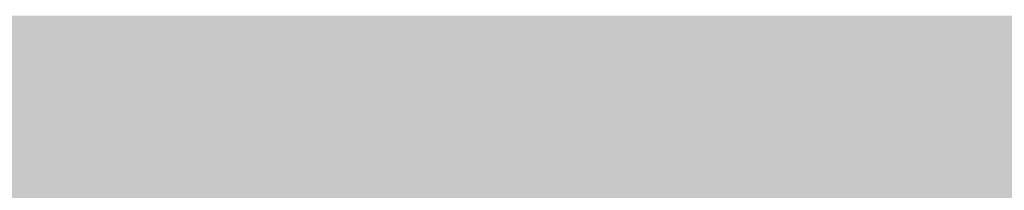
# Model space of a CAD drawing. Units: feet. Extents: x 3168 to 4724, y 827 to 1477.
# Tile 229 of 256: x 3379.08 to 3382.882, y 1098.344 to 1099.001. Entities that reach past the tile are written whole.
import ezdxf

# ---------------------------------------------------------------- set-up
doc = ezdxf.new("R2010")
doc.units = ezdxf.units.FT
doc.layers.add('A-ELEV', color=7, linetype='Continuous', lineweight=35)
doc.layers.add('A-ELEV-PATT', color=8, linetype='Continuous', lineweight=13)

msp = doc.modelspace()

# ---------------------------------------------------------------- hatches: boundary and pattern name
at = {"layer": 'A-ELEV-PATT'}
h = msp.add_hatch(color=256, dxfattribs=at)
h.dxf.hatch_style = 1
edge = h.paths.add_edge_path()
edge.add_ellipse((3552.9058, 979.2201), major_axis=(36.7449, 0), ratio=0.4848485, start_angle=0, end_angle=360)
edge = h.paths.add_edge_path()
edge.add_ellipse((3559.8916, 929.2523), major_axis=(36.7449, 0), ratio=0.4848485, start_angle=0, end_angle=360)
edge = h.paths.add_edge_path()
edge.add_line((3299.3168, 1198.6061), (3479.9167, 1198.6061))
edge.add_line((3479.9167, 1198.6061), (3479.9167, 1209.8686))
edge.add_spline(control_points=[(3479.9167, 1209.8686), (3464.3012, 1209.8686), (3448.6856, 1209.8686), (3410.9491, 1209.8686), (3388.8282, 1209.8686), (3355.6469, 1209.8686), (3344.5864, 1209.8686), (3327.9957, 1209.8686), (3322.4655, 1209.8686), (3314.1702, 1209.8686), (3311.4051, 1209.8686), (3307.2574, 1209.8686), (3305.8748, 1209.8686), (3303.801, 1209.8686), (3303.1097, 1209.8686), (3302.0728, 1209.8686), (3301.7272, 1209.8686), (3301.2087, 1209.8686), (3301.0359, 1209.8686), (3300.7767, 1209.8686), (3300.6903, 1209.8686), (3300.5606, 1209.8686), (3300.5174, 1209.8686), (3300.4526, 1209.8686), (3300.431, 1209.8686), (3300.3986, 1209.8686), (3300.3878, 1209.8686), (3300.3662, 1209.8686), (3300.3457, 1209.8686), (3300.3455, 1209.8686), (3300.3455, 1209.8686), (3300.3433, 1209.8686), (3300.3411, 1209.8686), (3300.3379, 1209.8686), (3300.3368, 1209.8686), (3300.3339, 1209.8686), (3300.3321, 1209.8686), (3300.3255, 1209.8686), (3300.3207, 1209.8686), (3300.3109, 1209.8686), (3300.306, 1209.8686), (3300.2905, 1209.8686), (3300.28, 1209.8686), (3300.2324, 1209.8688), (3300.1953, 1209.869), (3299.9511, 1209.8706), (3299.7448, 1209.8743), (3299.4368, 1209.8833), (3299.3344, 1209.8868), (3299.1811, 1209.8929), (3299.13, 1209.8951), (3298.6522, 1209.9168), (3298.2295, 1209.9457), (3297.6016, 1210.0024), (3297.3934, 1210.0235), (3297.0827, 1210.0583), (3296.9793, 1210.0705), (3296.293, 1210.1549), (3295.7181, 1210.2434), (3294.8687, 1210.3989), (3294.5877, 1210.4545), (3294.1693, 1210.5433), (3294.0304, 1210.5739), (3291.7071, 1211.1012), (3289.6536, 1211.8134), (3285.7763, 1213.564), (3283.9514, 1214.6035), (3280.5122, 1216.9801), (3278.8972, 1218.3176), (3276.3799, 1220.8295), (3275.416, 1221.9177), (3274.0393, 1223.7077), (3273.581, 1224.3495), (3273.1432, 1225.0163)], knot_values=[39.119033, 39.119033, 39.119033, 39.119033, 39.286353, 39.286353, 39.523379, 39.523379, 39.641892, 39.641892, 39.701148, 39.701148, 39.730777, 39.730777, 39.745591, 39.745591, 39.752998, 39.752998, 39.756701, 39.756701, 39.758553, 39.758553, 39.759479, 39.759479, 39.759942, 39.759942, 39.760173, 39.760173, 39.760289, 39.760289, 39.760405, 39.760405, 39.760463, 39.760463, 39.763389, 39.763389, 39.764851, 39.764851, 39.767304, 39.767304, 39.773825, 39.773825, 39.78057, 39.78057, 39.79477, 39.79477, 39.845194, 39.845194, 40.126715, 40.126715, 40.267476, 40.267476, 40.337856, 40.337856, 40.927023, 40.927023, 41.221606, 41.221606, 41.368898, 41.368898, 42.202622, 42.202622, 42.619485, 42.619485, 42.827916, 42.827916, 46.118323, 46.118323, 49.408731, 49.408731, 52.699139, 52.699139, 54.927489, 54.927489, 56.104228, 56.104228, 56.104228, 56.104228], weights=[1, 1, 1, 1, 1, 1, 1, 1, 1, 1, 1, 1, 1, 1, 1, 1, 1, 1, 1, 1, 1, 1, 1, 1, 1, 1, 1, 1, 1, 1, 1, 1, 1, 1, 1, 1, 1, 1, 1, 1, 1, 1, 1, 1, 1, 1, 1, 1, 1, 1, 1, 1, 1, 1, 1, 1, 1, 1, 1, 1, 1, 1, 1, 1, 1, 1, 1, 1, 1, 1, 1, 1, 1, 1], degree=3, periodic=0)
edge.add_line((3273.1432, 1225.0163), (3273.1432, 1099.0163))
edge.add_line((3273.1432, 1099.0163), (3299.3168, 1099.0163))
edge.add_line((3299.3168, 1099.0163), (3299.3168, 1198.6061))
edge = h.paths.add_edge_path()
edge.add_line((3304.7584, 1324.1581), (3479.9167, 1324.1581))
edge.add_line((3479.9167, 1324.1581), (3479.9167, 1335.7146))
edge.add_line((3479.9167, 1335.7146), (3269.1616, 1335.7146))
edge.add_spline(control_points=[(3269.1616, 1335.7146), (3264.0242, 1335.7146), (3258.3641, 1328.9582), (3259.2643, 1323.9003)], knot_values=[0, 0, 0, 0, 15.412191, 15.412191, 15.412191, 15.412191], degree=3, periodic=0)
edge.add_line((3259.2643, 1323.9003), (3265.5168, 1288.7691))
edge.add_line((3265.5168, 1288.7691), (3275.2651, 1261.5456))
edge.add_line((3275.2651, 1261.5456), (3304.7584, 1261.5456))
edge.add_line((3304.7584, 1261.5456), (3304.7584, 1324.1581))
h = msp.add_hatch(color=256, dxfattribs=at)
h.dxf.hatch_style = 1
h.paths.add_polyline_path([(3384.5252, 1099.0163), (3335.0292, 1099.0163), (3299.3168, 1099.0163), (3273.1432, 1099.0163), (3217.5654, 1099.0163), (3168.0693, 827.1163), (3335.0292, 827.1163)])

# ---------------------------------------------------------------- linework, layer by layer
at = {"layer": 'A-ELEV'}
msp.add_open_spline([(3808.5202, 1099.0163), (3808.5202, 1141.4132), (3808.5202, 1183.8102), (3808.5202, 1226.6353), (3808.5202, 1227.0636), (3808.5202, 1227.4918), (3811.4919, 1248.9947), (3814.4635, 1270.4975), (3817.4652, 1292.2176), (3817.4952, 1292.4348), (3817.5253, 1292.652), (3817.5728, 1310.1067), (3817.6203, 1327.5615), (3817.6679, 1345.0163), (3817.6679, 1345.458), (3817.6679, 1345.8996), (3817.6679, 1346.456), (3817.6679, 1346.5708), (3817.6679, 1346.7529), (3817.6679, 1346.8201), (3817.6679, 1346.9349), (3817.6679, 1346.9823), (3817.6679, 1347.0386), (3817.6679, 1347.0474), (3817.6679, 1347.0737), (3817.6679, 1347.0593), (3817.6679, 1347.0615), (3817.6679, 1347.0627), (3817.6679, 1347.066), (3817.6679, 1347.0683), (3817.6679, 1347.075), (3817.6679, 1347.0795), (3817.6678, 1347.0929), (3817.6678, 1347.1019), (3817.6678, 1347.1288), (3817.6677, 1347.1467), (3817.6674, 1347.2004), (3817.6672, 1347.2362), (3817.6661, 1347.3434), (3817.665, 1347.4147), (3817.6608, 1347.6281), (3817.6566, 1347.7697), (3817.64, 1348.1925), (3817.6235, 1348.4716), (3817.5591, 1349.3001), (3817.4961, 1349.8406), (3817.2554, 1351.4242), (3817.0263, 1352.4288), (3816.3069, 1354.8889), (3815.7437, 1356.2687), (3814.464, 1358.8192), (3813.7464, 1359.991), (3812.1958, 1362.1723), (3811.3622, 1363.1821), (3809.5888, 1365.069), (3808.6488, 1365.9461), (3806.6543, 1367.5796), (3805.5997, 1368.3362), (3803.3529, 1369.7223), (3802.1605, 1370.3524), (3799.6008, 1371.4536), (3798.2327, 1371.9255), (3795.2801, 1372.6346), (3793.6931, 1372.8721), (3791.8694, 1372.9265), (3791.7409, 1372.9292), (3791.3534, 1372.9341), (3791.0927, 1372.9329), (3790.3041, 1372.9151), (3789.7695, 1372.8842), (3789.2092, 1372.8302), (3789.1906, 1372.8284), (3789.1349, 1372.8229), (3789.0977, 1372.8191), (3789.0484, 1372.814), (3789.0364, 1372.8127), (3789.0003, 1372.8089), (3788.9761, 1372.8063), (3788.9494, 1372.8034), (3788.9468, 1372.8031), (3788.9426, 1372.8027), (3788.941, 1372.8025), (3788.9386, 1372.8022), (3788.9378, 1372.8021), (3788.9354, 1372.8019), (3788.8675, 1372.7944), (3788.7569, 1372.7822), (3788.7015, 1372.7761), (3788.5355, 1372.7579), (3788.4249, 1372.7457), (3788.0929, 1372.7092), (3787.8715, 1372.6848), (3787.2075, 1372.6118), (3786.7648, 1372.5631), (3785.4368, 1372.417), (3784.5515, 1372.3196), (3781.8954, 1372.0274), (3780.1247, 1371.8327), (3774.8126, 1371.2483), (3771.2713, 1370.8587), (3760.6471, 1369.69), (3753.5643, 1368.9109), (3732.316, 1366.5735), (3718.1504, 1365.0152), (3694.0068, 1362.3593), (3684.0287, 1361.2617), (3674.0506, 1360.1641), (3664.6007, 1360.1641), (3655.1508, 1360.1641), (3626.8011, 1360.1641), (3607.9013, 1360.1641), (3551.2019, 1360.1641), (3513.4023, 1360.1641), (3467.7252, 1360.1641), (3459.8476, 1360.1641), (3436.2149, 1360.1641), (3420.4597, 1360.1641), (3373.1943, 1360.1641), (3341.6839, 1360.1641), (3302.8482, 1360.1641), (3295.5227, 1360.1641), (3286.0383, 1360.1641), (3283.8794, 1360.1641), (3277.4026, 1360.1641), (3273.0848, 1360.1641), (3267.7329, 1360.1641), (3266.6988, 1360.1641), (3263.5965, 1360.1641), (3261.5284, 1360.1641), (3259.2369, 1360.1641), (3259.0137, 1360.1641), (3258.344, 1360.1641), (3257.8975, 1360.1641), (3257.431, 1360.1641), (3257.411, 1360.1641), (3257.3706, 1360.1641), (3257.3755, 1360.1641), (3257.3746, 1360.1641), (3257.3739, 1360.1641), (3257.372, 1360.1641), (3257.3706, 1360.1641), (3257.3667, 1360.1641), (3257.364, 1360.1641), (3257.3561, 1360.1641), (3257.3508, 1360.164), (3257.335, 1360.164), (3257.3244, 1360.164), (3257.2928, 1360.1639), (3257.2717, 1360.1638), (3257.2084, 1360.1634), (3257.1663, 1360.163), (3257.0402, 1360.1614), (3256.9563, 1360.1598), (3256.7055, 1360.1534), (3256.5392, 1360.147), (3256.0436, 1360.1219), (3255.7173, 1360.0971), (3254.7524, 1360.0005), (3254.128, 1359.9065), (3252.1801, 1359.5253), (3250.9416, 1359.144), (3248.6702, 1358.2433), (3247.6357, 1357.7238), (3245.7326, 1356.6035), (3244.8634, 1356.0021), (3243.2531, 1354.7429), (3242.512, 1354.0847), (3240.7511, 1352.3448), (3239.801, 1351.2296), (3238.0878, 1348.8724), (3237.3247, 1347.6304), (3235.9825, 1344.9716), (3235.4022, 1343.5549), (3234.5911, 1340.8155), (3234.3109, 1339.5435), (3233.9765, 1336.8026), (3233.9221, 1335.3309), (3234.1489, 1332.5913), (3234.3495, 1331.3672), (3234.7199, 1329.9994), (3234.7524, 1329.8834), (3234.8536, 1329.5348), (3234.9259, 1329.3017), (3235.0248, 1329.0026), (3235.0469, 1328.9369), (3235.0776, 1328.8472), (3235.0859, 1328.8232), (3235.1109, 1328.7511), (3235.1278, 1328.703), (3235.148, 1328.6462), (3235.1511, 1328.6376), (3235.1561, 1328.6235), (3235.1581, 1328.618), (3235.1602, 1328.612), (3235.1656, 1328.5969), (3235.1801, 1328.5565), (3235.1903, 1328.5281), (3235.2208, 1328.4429), (3235.2411, 1328.3862), (3235.3021, 1328.2159), (3235.3427, 1328.1023), (3235.4647, 1327.7617), (3235.546, 1327.5346), (3235.79, 1326.8534), (3235.9526, 1326.3992), (3236.4405, 1325.0367), (3236.7657, 1324.1284), (3237.7415, 1321.4034), (3238.392, 1319.5868), (3240.3435, 1314.1369), (3241.6445, 1310.5036), (3245.5476, 1299.6037), (3248.1496, 1292.3371), (3255.9557, 1270.5374), (3261.1598, 1256.0042), (3267.3876, 1238.612), (3268.4114, 1235.7529), (3269.5104, 1232.6839), (3269.5856, 1232.4739), (3269.7066, 1232.1359), (3269.7524, 1232.0079), (3269.8273, 1231.7987), (3269.8564, 1231.7176), (3269.9063, 1231.5781), (3269.9272, 1231.5198), (3269.9725, 1231.3934), (3269.9968, 1231.3254), (3270.0265, 1231.2425), (3270.0318, 1231.2277), (3270.0403, 1231.204), (3270.0392, 1231.207), (3270.0394, 1231.2066), (3270.0394, 1231.2064), (3270.0396, 1231.2058), (3270.0398, 1231.2055), (3270.0402, 1231.2043), (3270.0404, 1231.2036), (3270.0413, 1231.2013), (3270.0418, 1231.1998), (3270.0434, 1231.1953), (3270.0445, 1231.1922), (3270.0478, 1231.1832), (3270.0499, 1231.1771), (3270.0564, 1231.159), (3270.0608, 1231.147), (3270.0739, 1231.1108), (3270.0826, 1231.0867), (3270.1089, 1231.0144), (3270.1266, 1230.9663), (3270.1799, 1230.8225), (3270.2159, 1230.7269), (3270.3253, 1230.4415), (3270.4, 1230.2528), (3270.6292, 1229.6914), (3270.7889, 1229.3235), (3271.2865, 1228.2383), (3271.6431, 1227.5398), (3272.7759, 1225.5153), (3273.6142, 1224.2605), (3275.416, 1221.9177), (3276.3799, 1220.8295), (3278.8972, 1218.3176), (3280.5122, 1216.9801), (3283.9514, 1214.6035), (3285.7763, 1213.564), (3289.6536, 1211.8134), (3291.7071, 1211.1012), (3294.0304, 1210.5739), (3294.1693, 1210.5433), (3294.5877, 1210.4545), (3294.8687, 1210.3989), (3295.7181, 1210.2434), (3296.293, 1210.1549), (3296.9793, 1210.0705), (3297.0827, 1210.0583), (3297.3934, 1210.0235), (3297.6016, 1210.0024), (3298.2295, 1209.9457), (3298.6522, 1209.9168), (3299.13, 1209.8951), (3299.1811, 1209.8929), (3299.3344, 1209.8868), (3299.4368, 1209.8833), (3299.7448, 1209.8743), (3299.9511, 1209.8706), (3300.1953, 1209.869), (3300.2324, 1209.8688), (3300.28, 1209.8686), (3300.2905, 1209.8686), (3300.306, 1209.8686), (3300.3109, 1209.8686), (3300.3207, 1209.8686), (3300.3255, 1209.8686), (3300.3321, 1209.8686), (3300.3339, 1209.8686), (3300.3368, 1209.8686), (3300.3379, 1209.8686), (3300.3411, 1209.8686), (3300.3433, 1209.8686), (3300.3455, 1209.8686), (3300.3455, 1209.8686), (3300.3457, 1209.8686), (3300.3662, 1209.8686), (3300.3878, 1209.8686), (3300.3986, 1209.8686), (3300.431, 1209.8686), (3300.4526, 1209.8686), (3300.5174, 1209.8686), (3300.5606, 1209.8686), (3300.6903, 1209.8686), (3300.7767, 1209.8686), (3301.0359, 1209.8686), (3301.2087, 1209.8686), (3301.7272, 1209.8686), (3302.0728, 1209.8686), (3303.1097, 1209.8686), (3303.801, 1209.8686), (3305.8748, 1209.8686), (3307.2574, 1209.8686), (3311.4051, 1209.8686), (3314.1702, 1209.8686), (3322.4655, 1209.8686), (3327.9957, 1209.8686), (3344.5864, 1209.8686), (3355.6469, 1209.8686), (3388.8282, 1209.8686), (3410.9491, 1209.8686), (3477.3119, 1209.8686), (3521.5537, 1209.8686), (3566.8362, 1209.8686), (3567.8769, 1209.8686), (3570.999, 1209.8686), (3573.0804, 1209.8686), (3575.7814, 1209.8686), (3576.4009, 1209.8686), (3577.2958, 1209.8686), (3577.5712, 1209.8686), (3578.3971, 1209.8686), (3578.9478, 1209.8686), (3579.7565, 1209.8686), (3580.0145, 1209.8686), (3580.3427, 1209.8686), (3580.3269, 1209.8686), (3580.3272, 1209.8686), (3580.3273, 1209.8686), (3580.3278, 1209.8686), (3580.3281, 1209.8686), (3580.329, 1209.8686), (3580.3296, 1209.8686), (3580.3314, 1209.8686), (3580.3327, 1209.8686), (3580.3363, 1209.8686), (3580.3388, 1209.8686), (3580.3461, 1209.8686), (3580.351, 1209.8686), (3580.3657, 1209.8685), (3580.3754, 1209.8685), (3580.4048, 1209.8684), (3580.4244, 1209.8684), (3580.4832, 1209.8681), (3580.5224, 1209.8678), (3580.6404, 1209.8666), (3580.7192, 1209.8655), (3580.9563, 1209.8608), (3581.1152, 1209.8561), (3581.5942, 1209.8372), (3581.9164, 1209.8183), (3582.8899, 1209.7424), (3583.548, 1209.6662), (3585.5318, 1209.3606), (3586.8672, 1209.0539), (3589.4715, 1208.2525), (3590.7402, 1207.7579), (3591.9955, 1207.1588), (3592.0578, 1207.1287), (3592.2442, 1207.038), (3592.3677, 1206.9766), (3592.7353, 1206.7904), (3592.9768, 1206.6631), (3593.2445, 1206.5164), (3593.2747, 1206.4998), (3593.3651, 1206.4498), (3593.4251, 1206.4163), (3593.6043, 1206.3153), (3593.7227, 1206.2472), (3593.8572, 1206.1684), (3593.8744, 1206.1583), (3593.9257, 1206.128), (3593.9599, 1206.1078), (3594.0621, 1206.0469), (3594.1298, 1206.0061), (3594.2084, 1205.9582), (3594.2197, 1205.9513), (3594.2534, 1205.9307), (3594.2758, 1205.9169), (3594.343, 1205.8755), (3594.3876, 1205.8479), (3594.4336, 1205.819), (3594.4353, 1205.818), (3594.4402, 1205.8149), (3594.4435, 1205.8129), (3594.4471, 1205.8106), (3594.4475, 1205.8103), (3594.4487, 1205.8096), (3594.4495, 1205.8091), (3594.4504, 1205.8086), (3594.4505, 1205.8085), (3594.4506, 1205.8084), (3594.4674, 1205.7979), (3594.4933, 1205.7817), (3594.5062, 1205.7736), (3594.545, 1205.7492), (3594.5709, 1205.733), (3594.6485, 1205.6844), (3594.7002, 1205.652), (3594.8554, 1205.5547), (3594.9589, 1205.4898), (3595.2694, 1205.2953), (3595.4763, 1205.1656), (3596.0972, 1204.7765), (3596.5111, 1204.5171), (3597.7528, 1203.7388), (3598.5807, 1203.22), (3601.0642, 1201.6636), (3602.7198, 1200.6259), (3607.6868, 1197.513), (3610.9981, 1195.4377), (3620.932, 1189.2119), (3627.5546, 1185.0614), (3647.4225, 1172.6097), (3660.6678, 1164.3086), (3700.4035, 1139.4053), (3726.894, 1122.8031), (3757.2057, 1103.8061), (3761.027, 1101.4112), (3764.8482, 1099.0163), (3745.3283, 1099.0163), (3725.8083, 1099.0163), (3706.2884, 1099.0163), (3706.2884, 1108.4532), (3706.2884, 1117.8902), (3706.2884, 1127.3271), (3710.7508, 1127.3271), (3715.2131, 1127.3271), (3719.6755, 1127.3271)], degree=3, knots=[0, 0, 0, 0, 0.982037, 0.982037, 0.991957, 0.991957, 0.991957, 1.966522, 1.966522, 1.976367, 1.976367, 1.976367, 2.976367, 2.976367, 2.976367, 3.00169, 3.00169, 3.008272, 3.008272, 3.012129, 3.012129, 3.014851, 3.014851, 3.015353, 3.015353, 3.016359, 3.016359, 3.017365, 3.017365, 3.019376, 3.019376, 3.023398, 3.023398, 3.031442, 3.031442, 3.047531, 3.047531, 3.079708, 3.079708, 3.144063, 3.144063, 3.272772, 3.272772, 3.53019, 3.53019, 4.045026, 4.045026, 5.074698, 5.074698, 6.700878, 6.700878, 8.327058, 8.327058, 9.953238, 9.953238, 11.579418, 11.579418, 13.205598, 13.205598, 14.831778, 14.831778, 16.457958, 16.457958, 18.084138, 18.084138, 18.206872, 18.206872, 18.45234, 18.45234, 18.943275, 18.943275, 18.960093, 18.960093, 18.993729, 18.993729, 19.00461, 19.00461, 19.026374, 19.026374, 19.028737, 19.028737, 19.03018, 19.03018, 19.030897, 19.030897, 19.032332, 19.032332, 19.033766, 19.033766, 19.036636, 19.036636, 19.042374, 19.042374, 19.053851, 19.053851, 19.076805, 19.076805, 19.122714, 19.122714, 19.21453, 19.21453, 19.398163, 19.398163, 19.765429, 19.765429, 20.024128, 20.024128, 20.024128, 20.092031, 20.092031, 20.227836, 20.227836, 20.499446, 20.499446, 20.556051, 20.556051, 20.66926, 20.66926, 20.895678, 20.895678, 20.948316, 20.948316, 20.963829, 20.963829, 20.994855, 20.994855, 21.002285, 21.002285, 21.017146, 21.017146, 21.01875, 21.01875, 21.021959, 21.021959, 21.022102, 21.022102, 21.022249, 21.022249, 21.022708, 21.022708, 21.023627, 21.023627, 21.025464, 21.025464, 21.029138, 21.029138, 21.036486, 21.036486, 21.051183, 21.051183, 21.080575, 21.080575, 21.139361, 21.139361, 21.256932, 21.256932, 21.492073, 21.492073, 21.962356, 21.962356, 23.01002, 23.01002, 24.057684, 24.057684, 25.105348, 25.105348, 26.153011, 26.153011, 27.776787, 27.776787, 29.400562, 29.400562, 31.024337, 31.024337, 32.278801, 32.278801, 33.533265, 33.533265, 34.467568, 34.467568, 34.553971, 34.553971, 34.726776, 34.726776, 34.775309, 34.775309, 34.793079, 34.793079, 34.82862, 34.82862, 34.834979, 34.834979, 34.839039, 34.839039, 34.839411, 34.839411, 34.840285, 34.840285, 34.842034, 34.842034, 34.845531, 34.845531, 34.852525, 34.852525, 34.866512, 34.866512, 34.894488, 34.894488, 34.950439, 34.950439, 35.062342, 35.062342, 35.286147, 35.286147, 35.733758, 35.733758, 35.821815, 35.821815, 35.828283, 35.828283, 35.832225, 35.832225, 35.834724, 35.834724, 35.836521, 35.836521, 35.838617, 35.838617, 35.839073, 35.839073, 35.839345, 35.839345, 35.839617, 35.839617, 35.840161, 35.840161, 35.841249, 35.841249, 35.843425, 35.843425, 35.847778, 35.847778, 35.856482, 35.856482, 35.873891, 35.873891, 35.908709, 35.908709, 35.978345, 35.978345, 36.117617, 36.117617, 36.396161, 36.396161, 36.953248, 36.953248, 38.067423, 38.067423, 40.295772, 40.295772, 42.524122, 42.524122, 45.81453, 45.81453, 49.104937, 49.104937, 52.395345, 52.395345, 52.603776, 52.603776, 53.020639, 53.020639, 53.854363, 53.854363, 54.001655, 54.001655, 54.296238, 54.296238, 54.885405, 54.885405, 54.955785, 54.955785, 55.096546, 55.096546, 55.378067, 55.378067, 55.42849, 55.42849, 55.442691, 55.442691, 55.449436, 55.449436, 55.455957, 55.455957, 55.458409, 55.458409, 55.459872, 55.459872, 55.462798, 55.462798, 55.462856, 55.462856, 55.462972, 55.462972, 55.463088, 55.463088, 55.463319, 55.463319, 55.463782, 55.463782, 55.464708, 55.464708, 55.46656, 55.46656, 55.470263, 55.470263, 55.47767, 55.47767, 55.492484, 55.492484, 55.522112, 55.522112, 55.581369, 55.581369, 55.699882, 55.699882, 55.936907, 55.936907, 56.410959, 56.410959, 56.42211, 56.42211, 56.444413, 56.444413, 56.451051, 56.451051, 56.454001, 56.454001, 56.459901, 56.459901, 56.462666, 56.462666, 56.463418, 56.463418, 56.464171, 56.464171, 56.465675, 56.465675, 56.468684, 56.468684, 56.474702, 56.474702, 56.486738, 56.486738, 56.51081, 56.51081, 56.558955, 56.558955, 56.655243, 56.655243, 56.847821, 56.847821, 57.232975, 57.232975, 58.003284, 58.003284, 59.543901, 59.543901, 62.625137, 62.625137, 68.787607, 68.787607, 74.950078, 74.950078, 75.27336, 75.27336, 75.919923, 75.919923, 77.213051, 77.213051, 77.377769, 77.377769, 77.707206, 77.707206, 78.366079, 78.366079, 78.462532, 78.462532, 78.655436, 78.655436, 79.041245, 79.041245, 79.105735, 79.105735, 79.234714, 79.234714, 79.492672, 79.492672, 79.502197, 79.502197, 79.521249, 79.521249, 79.523534, 79.523534, 79.528103, 79.528103, 79.528682, 79.528682, 79.528885, 79.528885, 79.529089, 79.529089, 79.529495, 79.529495, 79.530308, 79.530308, 79.531935, 79.531935, 79.535187, 79.535187, 79.541693, 79.541693, 79.554704, 79.554704, 79.580725, 79.580725, 79.632769, 79.632769, 79.736856, 79.736856, 79.94503, 79.94503, 80.361377, 80.361377, 80.421435, 80.421435, 80.421435, 81.421435, 81.421435, 81.421435, 82.421435, 82.421435, 82.421435, 83.421435, 83.421435, 83.421435, 83.421435], dxfattribs=at)

doc.saveas('drawing.dxf')
